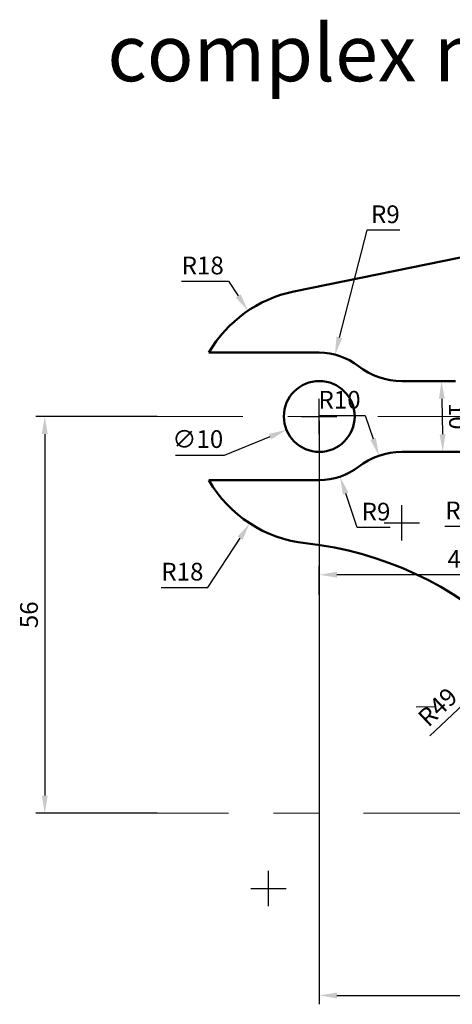
# Model space of a CAD drawing. Units: millimetres. Extents: x 59 to 241, y 36 to 183.
# Tile 1 of 2: x 59 to 120, y 44 to 183. Entities that reach past the tile are written whole.
import ezdxf

# ---------------------------------------------------------------- set-up
doc = ezdxf.new("R2010")
doc.units = ezdxf.units.MM
doc.linetypes.add('CENTER', pattern=[50.8, 31.75, -6.35, 6.35, -6.35])
for name, color, linetype, lineweight in [('M-CNTR', 1, 'CENTER', 18), ('M-DIMS', 2, 'Continuous', 25), ('M-OUTL', 7, 'Continuous', 50), ('M-TEXT', 3, 'Continuous', 25)]:
    doc.layers.add(name, color=color, linetype=linetype, lineweight=lineweight)
doc.styles.get("Standard").update_dxf_attribs({"font": 'arial.ttf'})
doc.dimstyles.new('ISO-25', dxfattribs={"dimtxt": 2.5, "dimasz": 2.5, "dimexe": 1.25, "dimexo": 0.625, "dimtad": 1, "dimtoh": 1, "dimdec": 0, "dimtxsty": 'Standard', "dimcen": 2.5, "dimadec": 0, "dimazin": 0, "dimtfac": 1, "dimtdec": 0, "dimtofl": 0, "dimtmove": 0, "dimatfit": 3, "dimfxl": 1, "dimarcsym": 0})

# ---------------------------------------------------------------- blocks, each defined once
blk = doc.blocks.new('*D1')
at = {"layer": 'Defpoints', "color": 0, "transparency": 16777216}
for p in [(79.18, 127.43), (62.7, 71.43), (79.18, 71.43)]:
    blk.add_point(p, dxfattribs=at)
at = {"layer": 'M-DIMS', "color": 0, "lineweight": -2, "transparency": 16777216}
for p, q in [((78.56, 127.43), (61.45, 127.43)), ((62.7, 124.93), (62.7, 73.93)), ((78.56, 71.43), (61.45, 71.43))]:
    blk.add_line(p, q, dxfattribs=at)
at = {"layer": 'M-DIMS', "color": 0, "transparency": 16777216}
for points in [[(62.28, 124.93), (63.12, 124.93), (62.7, 127.43)], [(62.28, 73.93), (63.12, 73.93), (62.7, 71.43)]]:
    blk.add_solid(points, dxfattribs=at)
at = {"layer": 'M-DIMS', "color": 0, "transparency": 16777216, "insert": (60.8, 99.43), "char_height": 2.5, "attachment_point": 5, "rotation": 90}
blk.add_mtext('56', dxfattribs=at)
blk = doc.blocks.new('*D2')
at = {"layer": 'Defpoints', "color": 0, "transparency": 16777216}
for p in [(101.46, 127.43), (161.46, 45.87), (161.46, 45.71)]:
    blk.add_point(p, dxfattribs=at)
at = {"layer": 'M-DIMS', "color": 0, "lineweight": -2, "transparency": 16777216}
for p, q in [((101.46, 126.8), (101.46, 44.46)), ((103.96, 45.71), (158.96, 45.71)), ((161.46, 45.24), (161.46, 44.46))]:
    blk.add_line(p, q, dxfattribs=at)
at = {"layer": 'M-DIMS', "color": 0, "transparency": 16777216}
for points in [[(103.96, 46.13), (103.96, 45.29), (101.46, 45.71)], [(158.96, 46.13), (158.96, 45.29), (161.46, 45.71)]]:
    blk.add_solid(points, dxfattribs=at)
at = {"layer": 'M-DIMS', "color": 0, "transparency": 16777216, "insert": (131.46, 47.61), "char_height": 2.5, "attachment_point": 5}
blk.add_mtext('60', dxfattribs=at)
blk = doc.blocks.new('*D9')
at = {"layer": 'Defpoints', "color": 0, "transparency": 16777216}
for p in [(91.41, 142.36), (101.46, 127.43)]:
    blk.add_point(p, dxfattribs=at)
at = {"layer": 'M-DIMS', "color": 0, "lineweight": -2, "transparency": 16777216}
for p, q in [((82.01, 146.51), (88.62, 146.51)), ((88.62, 146.51), (90.01, 144.44)), ((101.46, 124.93), (101.46, 129.93)), ((98.96, 127.43), (103.96, 127.43))]:
    blk.add_line(p, q, dxfattribs=at)
at = {"layer": 'M-DIMS', "color": 0, "transparency": 16777216}
blk.add_solid([(90.36, 144.67), (89.67, 144.2), (91.41, 142.36)], dxfattribs=at)
at = {"layer": 'M-DIMS', "color": 0, "transparency": 16777216, "insert": (85, 148.41), "char_height": 2.5, "attachment_point": 5}
blk.add_mtext('R18', dxfattribs=at)
blk = doc.blocks.new('*D10')
at = {"layer": 'Defpoints', "color": 0, "transparency": 16777216}
for p in [(103.68, 136.15), (101.46, 127.43)]:
    blk.add_point(p, dxfattribs=at)
at = {"layer": 'M-DIMS', "color": 0, "lineweight": -2, "transparency": 16777216}
for p, q in [((108.15, 153.74), (104.29, 138.57)), ((112.81, 153.74), (108.15, 153.74)), ((101.46, 124.93), (101.46, 129.93)), ((98.96, 127.43), (103.96, 127.43))]:
    blk.add_line(p, q, dxfattribs=at)
at = {"layer": 'M-DIMS', "color": 0, "transparency": 16777216}
blk.add_solid([(103.89, 138.68), (104.7, 138.47), (103.68, 136.15)], dxfattribs=at)
at = {"layer": 'M-DIMS', "color": 0, "transparency": 16777216, "insert": (110.79, 155.64), "char_height": 2.5, "attachment_point": 5}
blk.add_mtext('R9', dxfattribs=at)
blk = doc.blocks.new('*D12')
at = {"layer": 'Defpoints', "color": 0, "transparency": 16777216}
for p in [(106.09, 129.32), (96.83, 125.53)]:
    blk.add_point(p, dxfattribs=at)
at = {"layer": 'M-DIMS', "color": 0, "lineweight": -2, "transparency": 16777216}
for p, q in [((101.46, 124.93), (101.46, 129.93)), ((98.96, 127.43), (103.96, 127.43)), ((88.07, 121.94), (94.52, 124.59)), ((81.15, 121.94), (88.07, 121.94))]:
    blk.add_line(p, q, dxfattribs=at)
at = {"layer": 'M-DIMS', "color": 0, "transparency": 16777216}
blk.add_solid([(94.36, 124.97), (94.68, 124.2), (96.83, 125.53)], dxfattribs=at)
at = {"layer": 'M-DIMS', "color": 0, "transparency": 16777216, "insert": (84.3, 123.91), "char_height": 2.5, "attachment_point": 5}
blk.add_mtext('∅10', dxfattribs=at)
blk = doc.blocks.new('*D13')
at = {"layer": 'Defpoints', "color": 0, "transparency": 16777216}
for p in [(129.91, 94.46), (94.29, 60.81)]:
    blk.add_point(p, dxfattribs=at)
at = {"layer": 'M-DIMS', "color": 0, "lineweight": -2, "transparency": 16777216}
blk.add_line((117.07, 82.33), (128.09, 92.74), dxfattribs=at)
at = {"layer": 'M-DIMS', "color": 0, "transparency": 16777216}
blk.add_solid([(127.81, 93.05), (128.38, 92.44), (129.91, 94.46)], dxfattribs=at)
at = {"layer": 'M-DIMS', "color": 0, "transparency": 16777216, "insert": (118.39, 86.19), "char_height": 2.5, "attachment_point": 5, "rotation": 43.3695}
blk.add_mtext('R49', dxfattribs=at)
blk = doc.blocks.new('*D27')
at = {"layer": 'Defpoints', "color": 0, "transparency": 16777216}
for p in [(141.46, 127.43), (101.46, 105.09), (101.46, 101.65)]:
    blk.add_point(p, dxfattribs=at)
at = {"layer": 'M-DIMS', "color": 0, "lineweight": -2, "transparency": 16777216}
for p, q in [((141.46, 126.8), (141.46, 103.84)), ((101.46, 102.27), (101.46, 106.34)), ((138.96, 105.09), (103.96, 105.09))]:
    blk.add_line(p, q, dxfattribs=at)
at = {"layer": 'M-DIMS', "color": 0, "transparency": 16777216}
for points in [[(103.96, 105.51), (103.96, 104.68), (101.46, 105.09)], [(138.96, 105.51), (138.96, 104.68), (141.46, 105.09)]]:
    blk.add_solid(points, dxfattribs=at)
at = {"layer": 'M-DIMS', "color": 0, "transparency": 16777216, "insert": (121.46, 106.99), "char_height": 2.5, "attachment_point": 5}
blk.add_mtext('40', dxfattribs=at)
blk = doc.blocks.new('*D29')
at = {"layer": 'Defpoints', "color": 0, "transparency": 16777216}
for p in [(118.72, 132.43), (118.9, 122.43), (118.9, 122.43)]:
    blk.add_point(p, dxfattribs=at)
at = {"layer": 'M-DIMS', "color": 0, "lineweight": -2, "transparency": 16777216}
for p, q in [((119.35, 132.44), (119.97, 132.45)), ((118.77, 129.93), (118.86, 124.93)), ((119.53, 122.44), (120.15, 122.45))]:
    blk.add_line(p, q, dxfattribs=at)
at = {"layer": 'M-DIMS', "color": 0, "transparency": 16777216}
for points in [[(119.18, 129.94), (118.35, 129.92), (118.72, 132.43)], [(119.28, 124.94), (118.44, 124.92), (118.9, 122.43)]]:
    blk.add_solid(points, dxfattribs=at)
at = {"layer": 'M-DIMS', "color": 0, "transparency": 16777216, "insert": (120.71, 127.46), "char_height": 2.5, "attachment_point": 5, "rotation": 271.0391}
blk.add_mtext('10', dxfattribs=at)
blk = doc.blocks.new('*D34')
at = {"layer": 'Defpoints', "color": 0, "transparency": 16777216}
for p in [(128.07, 96.31), (94.29, 60.81)]:
    blk.add_point(p, dxfattribs=at)
at = {"layer": 'M-DIMS', "color": 0, "lineweight": -2, "transparency": 16777216}
for p, q in [((148.34, 117.61), (129.79, 98.12)), ((154.94, 117.61), (148.34, 117.61)), ((94.29, 58.31), (94.29, 63.31)), ((91.79, 60.81), (96.79, 60.81))]:
    blk.add_line(p, q, dxfattribs=at)
at = {"layer": 'M-DIMS', "color": 0, "transparency": 16777216}
blk.add_solid([(129.49, 98.41), (130.1, 97.83), (128.07, 96.31)], dxfattribs=at)
at = {"layer": 'M-DIMS', "color": 0, "transparency": 16777216, "insert": (151.95, 119.51), "char_height": 2.5, "attachment_point": 5}
blk.add_mtext('R49', dxfattribs=at)
blk = doc.blocks.new('*D38')
at = {"layer": 'Defpoints', "color": 0, "transparency": 16777216}
for p in [(101.46, 127.43), (91.64, 112.34)]:
    blk.add_point(p, dxfattribs=at)
at = {"layer": 'M-DIMS', "color": 0, "lineweight": -2, "transparency": 16777216}
for p, q in [((101.46, 124.93), (101.46, 129.93)), ((98.96, 127.43), (103.96, 127.43)), ((85.74, 103.29), (90.27, 110.25)), ((79.14, 103.29), (85.74, 103.29))]:
    blk.add_line(p, q, dxfattribs=at)
at = {"layer": 'M-DIMS', "color": 0, "transparency": 16777216}
blk.add_solid([(89.92, 110.48), (90.62, 110.02), (91.64, 112.34)], dxfattribs=at)
at = {"layer": 'M-DIMS', "color": 0, "transparency": 16777216, "insert": (82.13, 105.2), "char_height": 2.5, "attachment_point": 5}
blk.add_mtext('R18', dxfattribs=at)
blk = doc.blocks.new('*D42')
at = {"layer": 'Defpoints', "color": 0, "transparency": 16777216}
for p in [(141.46, 127.43), (133.52, 117.77)]:
    blk.add_point(p, dxfattribs=at)
at = {"layer": 'M-DIMS', "color": 0, "lineweight": -2, "transparency": 16777216}
for p, q in [((141.46, 124.93), (141.46, 129.93)), ((138.96, 127.43), (143.96, 127.43)), ((128.73, 111.94), (131.94, 115.84)), ((119.2, 111.94), (128.73, 111.94))]:
    blk.add_line(p, q, dxfattribs=at)
at = {"layer": 'M-DIMS', "color": 0, "transparency": 16777216}
blk.add_solid([(131.61, 116.1), (132.26, 115.57), (133.52, 117.77)], dxfattribs=at)
at = {"layer": 'M-DIMS', "color": 0, "transparency": 16777216, "insert": (123.65, 113.84), "char_height": 2.5, "attachment_point": 5}
blk.add_mtext('R12.5', dxfattribs=at)
blk = doc.blocks.new('*D43')
at = {"layer": 'Defpoints', "color": 0, "transparency": 16777216}
for p in [(109.88, 121.89), (113.12, 112.43)]:
    blk.add_point(p, dxfattribs=at)
at = {"layer": 'M-DIMS', "color": 0, "lineweight": -2, "transparency": 16777216}
for p, q in [((101.34, 127.56), (107.93, 127.56)), ((107.93, 127.56), (109.06, 124.25)), ((113.12, 109.93), (113.12, 114.93)), ((110.62, 112.43), (115.62, 112.43))]:
    blk.add_line(p, q, dxfattribs=at)
at = {"layer": 'M-DIMS', "color": 0, "transparency": 16777216}
blk.add_solid([(109.46, 124.39), (108.67, 124.12), (109.88, 121.89)], dxfattribs=at)
at = {"layer": 'M-DIMS', "color": 0, "transparency": 16777216, "insert": (104.32, 129.46), "char_height": 2.5, "attachment_point": 5}
blk.add_mtext('R10', dxfattribs=at)
blk = doc.blocks.new('*D45')
at = {"layer": 'Defpoints', "color": 0, "transparency": 16777216}
for p in [(101.46, 127.43), (104.38, 118.91)]:
    blk.add_point(p, dxfattribs=at)
at = {"layer": 'M-DIMS', "color": 0, "lineweight": -2, "transparency": 16777216}
for p, q in [((101.46, 124.93), (101.46, 129.93)), ((98.96, 127.43), (103.96, 127.43)), ((106.83, 111.77), (105.19, 116.55)), ((111.49, 111.77), (106.83, 111.77))]:
    blk.add_line(p, q, dxfattribs=at)
at = {"layer": 'M-DIMS', "color": 0, "transparency": 16777216}
blk.add_solid([(105.58, 116.69), (104.79, 116.41), (104.38, 118.91)], dxfattribs=at)
at = {"layer": 'M-DIMS', "color": 0, "transparency": 16777216, "insert": (109.47, 113.67), "char_height": 2.5, "attachment_point": 5}
blk.add_mtext('R9', dxfattribs=at)

msp = doc.modelspace()

# ---------------------------------------------------------------- linework, layer by layer
at = {"layer": 'M-CNTR'}
for p, q in [((141.46, 127.43), (69.53, 127.43)), ((219.53, 86.43), (115.15, 86.43)), ((241.06, 71.43), (65.85, 71.43))]:
    msp.add_line(p, q, dxfattribs=at)
at = {"layer": 'M-OUTL'}
for p, q in [((136.26, 152.9), (97.86, 145.06)), ((101.46, 136.43), (85.87, 136.43)), ((113.12, 132.43), (120.69, 132.43)), ((113.12, 122.43), (124.69, 122.43)), ((101.46, 118.43), (85.87, 118.43))]:
    msp.add_line(p, q, dxfattribs=at)
msp.add_circle((101.46, 127.43), 5, dxfattribs=at)
for centre, radius, start, end in [((101.46, 127.43), 18, 101.537, 150), ((101.46, 127.43), 9, 52.1364, 90), ((113.12, 142.43), 10, 232.1364, 270), ((113.12, 112.43), 10, 90, 127.8636), ((101.46, 127.43), 9, 270, 307.8636), ((101.46, 127.43), 18, 210, 263.8599), ((94.29, 60.81), 49, 8.9813, 83.8599)]:
    msp.add_arc(centre, radius, start, end, dxfattribs=at)

# ---------------------------------------------------------------- texts
at = {"layer": 'M-TEXT', "insert": (71.54, 182.74), "char_height": 8, "attachment_point": 1}
msp.add_mtext_dynamic_manual_height_columns('complex mechanical bracket', width=206.9654, gutter_width=12.5, heights=[0], dxfattribs=at)

# ---------------------------------------------------------------- dimensions: what is measured, and where the dimension line sits
at = {"layer": 'M-DIMS'}
for center, mpoint, override, picture, middle in [((101.46, 127.43), (103.68, 136.15), {"dimclrd": 0, "dimclre": 0, "dimclrt": 0}, '*D10', (110.79, 153.74)), ((113.12, 112.43), (109.88, 121.89), {"dimdec": 0, "dimlfac": 1, "dimrnd": 0, "dimzin": 0, "dimdsep": 46, "dimlunit": 2}, '*D43', (104.32, 127.56)), ((101.46, 127.43), (91.64, 112.34), {"dimdec": 0, "dimlfac": 1, "dimrnd": 0, "dimzin": 0, "dimdsep": 46, "dimlunit": 2}, '*D38', (82.13, 103.29)), ((94.29, 60.81), (128.07, 96.31), {"dimdec": 0, "dimlfac": 1, "dimrnd": 0, "dimzin": 0, "dimdsep": 46, "dimlunit": 2}, '*D34', (151.95, 117.61)), ((94.29, 60.81), (129.91, 94.46), {"dimclrd": 0, "dimclre": 0, "dimclrt": 0}, '*D13', (119.7, 84.81))]:
    dim = msp.add_radius_dim(center=center, mpoint=mpoint, dimstyle='ISO-25', override=override, dxfattribs=at)
    dim.commit()
    dim.dimension.update_dxf_attribs({"geometry": picture, "text_midpoint": middle, "dimtype": 164})
for center, mpoint, override, picture, middle in [((101.46, 127.43), (91.41, 142.36), {"dimclrd": 0, "dimclre": 0, "dimclrt": 0}, '*D9', (85, 148.41)), ((101.46, 127.43), (104.38, 118.91), {"dimdec": 0, "dimlfac": 1, "dimrnd": 0, "dimzin": 0, "dimdsep": 46, "dimlunit": 2}, '*D45', (109.47, 113.67)), ((141.46, 127.43), (133.52, 117.77), {"dimdec": 1, "dimlfac": 1, "dimrnd": 0, "dimzin": 0, "dimdsep": 46, "dimlunit": 2}, '*D42', (123.65, 113.84))]:
    dim = msp.add_radius_dim(center=center, mpoint=mpoint, dimstyle='ISO-25', override=override, dxfattribs=at)
    dim.commit()
    dim.dimension.update_dxf_attribs({"geometry": picture, "text_midpoint": middle})
dim = msp.add_aligned_dim(p1=(118.72, 132.43), p2=(118.9, 122.43), distance=0, dimstyle='ISO-25', override={"dimclrd": 0, "dimclre": 0, "dimclrt": 0}, dxfattribs=at)
dim.commit()
dim.dimension.update_dxf_attribs({"geometry": '*D29', "text_midpoint": (120.71, 127.46)})
dim = msp.add_diameter_dim_2p(p1=(106.09, 129.32), p2=(96.83, 125.53), dimstyle='ISO-25', override={"dimclrd": 0, "dimclre": 0, "dimclrt": 0}, dxfattribs=at)
dim.commit()
dim.dimension.update_dxf_attribs({"geometry": '*D12', "text_midpoint": (84.3, 121.94), "dimtype": 163})
dim = msp.add_linear_dim(base=(62.7, 71.43), p1=(79.18, 127.43), p2=(79.18, 71.43), angle=90, dimstyle='ISO-25', override={"dimclrd": 0, "dimclre": 0, "dimclrt": 0}, dxfattribs=at)
dim.commit()
dim.dimension.update_dxf_attribs({"geometry": '*D1', "text_midpoint": (60.8, 99.43)})
for base, p1, p2, picture, middle in [((161.46, 45.71), (101.46, 127.43), (161.46, 45.87), '*D2', (131.46, 47.61)), ((101.46, 105.09), (141.46, 127.43), (101.46, 101.65), '*D27', (121.46, 106.99))]:
    dim = msp.add_linear_dim(base=base, p1=p1, p2=p2, dimstyle='ISO-25', override={"dimclrd": 0, "dimclre": 0, "dimclrt": 0}, dxfattribs=at)
    dim.commit()
    dim.dimension.update_dxf_attribs({"geometry": picture, "text_midpoint": middle})

doc.saveas('drawing.dxf')
